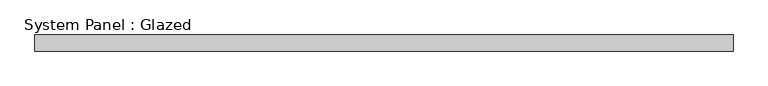
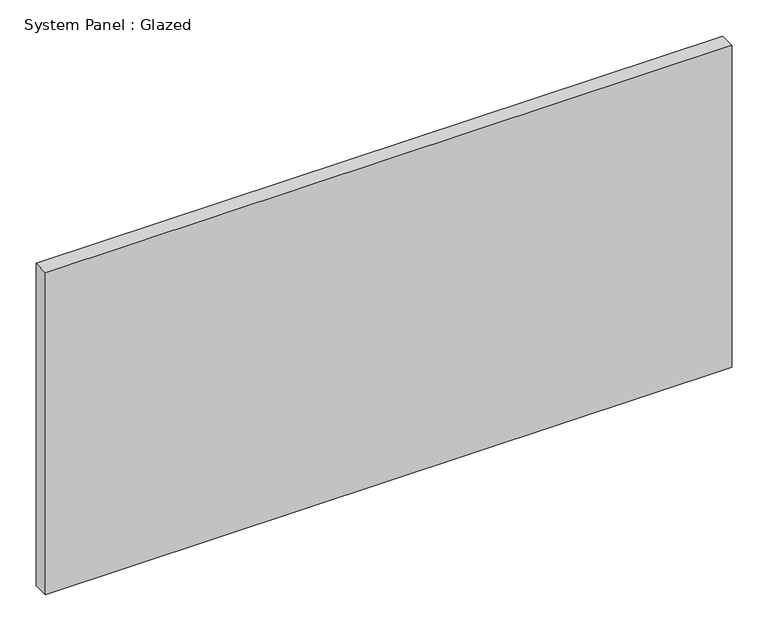
"""IFC4 building model written with IfcOpenShell, lengths in millimetres: plate geometry, System Panel : Glazed."""

from ifc_helpers import new_model, si_unit, origin, origin_with_axes, place, context, project, spatial, polyline, outline, extrude, source, transform, mapped, element, save


def system_panel_glazed_3a317166(model_context):
    return source(origin(), model_context, "Body", "SweptSolid", [
        extrude(outline(polyline([(550.3333332, 19.05), (-550.3333332, 19.05), (-550.3333332, 44.45), (550.3333332, 44.45), (550.3333332, 19.05)])), origin_with_axes(), (0.0, 0.0, 1.0), 546.1),
    ])


if __name__ == "__main__":
    model = new_model("IFC4")
    model_context = context("Model", 3, world=origin())
    ifc_project = project(units=[si_unit("LENGTHUNIT", "METRE", prefix="MILLI")], contexts=[model_context])
    site = spatial("IfcSite", under=ifc_project)
    building = spatial("IfcBuilding", under=site)
    placement = place(None, origin())
    system_panel_glazed_shape = system_panel_glazed_3a317166(model_context)
    element("IfcPlate", 1, ObjectType="System Panel : Glazed", at=placement, inside=building, context=model_context, shape_type="MappedRepresentation", body=[
        mapped(system_panel_glazed_shape, transform((0.0, 0.0, 0.0), x_axis=(1.0, 0.0, 0.0), y_axis=(0.0, 1.0, 0.0), z_axis=(0.0, 0.0, 1.0))),
    ])
    save(model, "model.ifc")

# Revit data of these elements
# Type "System Panel : Glazed"
#   Construction Type Id = "GSP4R"
#   Analytic Construction = "1/8 in Pilkington single glazing"
#   Visual Light Transmittance = 0.9
#   Solar Heat Gain Coefficient = 0.86
#   Heat Transfer Coefficient (U) = 1.18115 BTU/(h·ft²·°F)
#   Define Thermal Properties by = 1
# Element 1 (IfcPlate, "System Panel : Glazed")
#   Materials on its faces: "Glass"
# Materials
#   "Glass": class "Glass", colour RGB 0 128 192, transparency 0.75, Description = "Soda Lime Glass", Cost = 0
